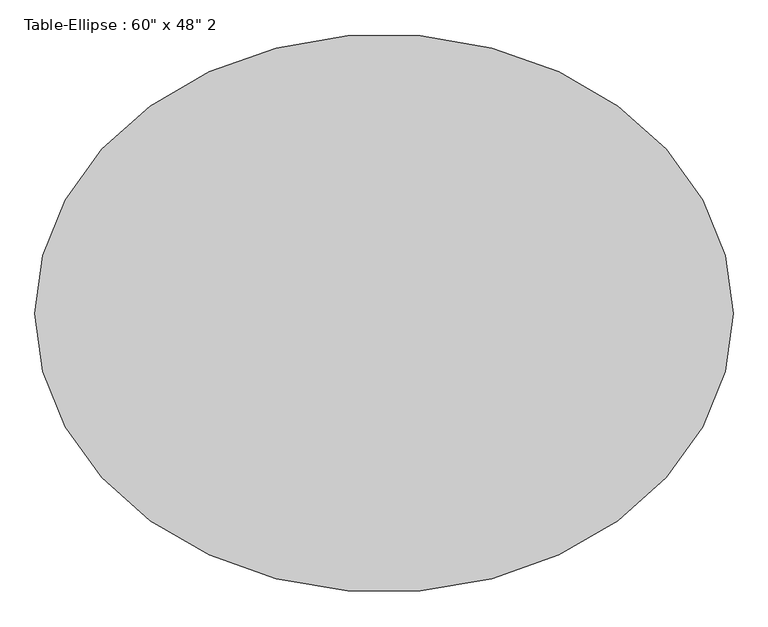
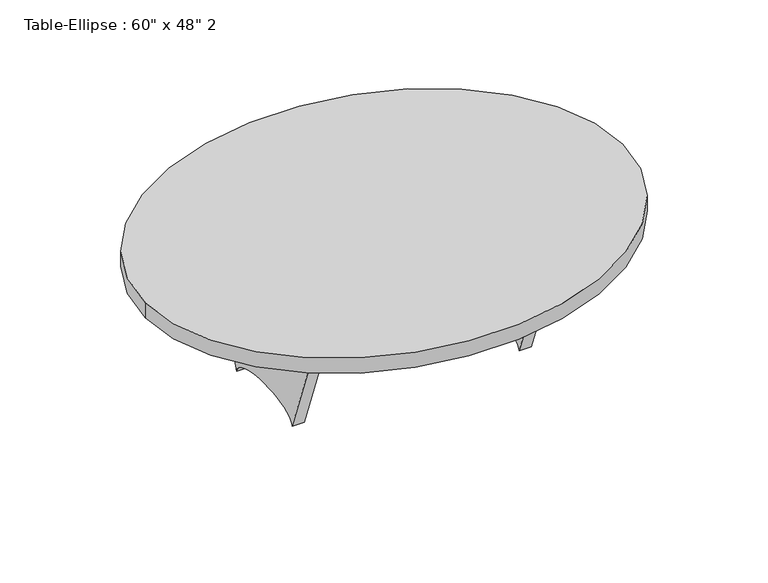
"""IFC4 building model written with IfcOpenShell, lengths in millimetres: furniture geometry."""

from ifc_helpers import new_model, si_unit, point, frame, origin, place, context, project, spatial, ellipse_curve, trimmed, source, transform, mapped, element, save
from ifc_brep_helpers import plane_surface, extruded_surface, advanced_brep


def furniture_c105135d(model_context):
    return source(origin(), model_context, "Body", "AdvancedBrep", [
        advanced_brep(
        [(-762.0, 0.0, 457.2), (762.0, 0.0, 457.2), (-762.0, 0.0, 406.4), (762.0, 0.0, 406.4)],
        [
            (0, 1, ellipse_curve(frame((0.0, 0.0, 457.2), z_axis=(0.0, 0.0, 1.0), x_axis=(1.0, 0.0, 0.0)), 762.0, 609.6)),
            (1, 0, ellipse_curve(frame((0.0, 0.0, 457.2), z_axis=(0.0, 0.0, 1.0), x_axis=(1.0, 0.0, 0.0)), 762.0, 609.6)),
            (2, 3, ellipse_curve(frame((0.0, 0.0, 406.4), z_axis=(0.0, 0.0, -1.0), x_axis=(1.0, 0.0, 0.0)), 762.0, 609.6)),
            (3, 2, ellipse_curve(frame((0.0, 0.0, 406.4), z_axis=(0.0, 0.0, -1.0), x_axis=(1.0, 0.0, 0.0)), 762.0, 609.6)),
            (0, 2),
            (3, 1),
        ],
        [
            plane_surface(frame((762.0, 0.0, 457.2), z_axis=(0.0, 0.0, 1.0), x_axis=(0.0, 1.0, 0.0))),
            plane_surface(frame((762.0, 0.0, 406.4), z_axis=(0.0, 0.0, -1.0), x_axis=(0.0, -1.0, 0.0))),
            extruded_surface(trimmed(ellipse_curve(frame((0.0, 0.0, 355.6), z_axis=(0.0, 0.0, 1.0), x_axis=(1.0, 0.0, 0.0)), 762.0, 609.6), [point((-762.0, 0.0, 355.6))], [point((762.0, 0.0, 355.6))], True, "CARTESIAN"), (0.0, 0.0, 50.799999999999955), 50.799999999999955),
            extruded_surface(trimmed(ellipse_curve(frame((0.0, 0.0, 355.6), z_axis=(0.0, 0.0, 1.0), x_axis=(1.0, 0.0, 0.0)), 762.0, 609.6), [point((762.0, 0.0, 355.6))], [point((-762.0, 0.0, 355.6))], True, "CARTESIAN"), (0.0, 0.0, 50.799999999999955), 50.799999999999955),
        ],
        [
            (0, [[1, 2]]),
            (1, [[3, 4]]),
            (2, [[-1, 5, -4, 6]]),
            (3, [[-2, -6, -3, -5]]),
        ],
    ),
        advanced_brep(
        [(-342.9, 304.8, 406.4), (-342.9, -304.8, 406.4), (-342.9, -152.4, 0.0), (-342.9, 152.4, 0.0), (-381.0, 304.8, 406.4), (-381.0, 152.4, 0.0), (-381.0, -152.4, 0.0), (-381.0, -304.8, 406.4)],
        [
            (0, 1),
            (1, 2),
            (2, 3, ellipse_curve(frame((-342.9, 0.0, 0.0), z_axis=(-1.0, 0.0, 0.0), x_axis=(0.0, 1.0, 0.0)), 152.4, 50.8)),
            (3, 0),
            (4, 5),
            (5, 6, ellipse_curve(frame((-381.0, 0.0, 0.0), z_axis=(1.0, 0.0, 0.0), x_axis=(0.0, 1.0, 0.0)), 152.4, 50.8)),
            (6, 7),
            (7, 4),
            (0, 4),
            (7, 1),
            (6, 2),
            (5, 3),
        ],
        [
            plane_surface(frame((-342.9, -304.8, 406.4), z_axis=(1.0, 0.0, 0.0), x_axis=(0.0, -1.0, 0.0))),
            plane_surface(frame((-381.0, -304.8, 406.4), z_axis=(-1.0, 0.0, 0.0), x_axis=(0.0, 1.0, 0.0))),
            plane_surface(frame((-342.9, 304.8, 406.4), z_axis=(0.0, 0.0, 1.0), x_axis=(-1.0, 0.0, 0.0))),
            plane_surface(frame((-342.9, -304.8, 406.4), z_axis=(0.0, -0.9363291775690403, -0.3511234415884029), x_axis=(-1.0, 0.0, 0.0))),
            extruded_surface(trimmed(ellipse_curve(frame((-419.1, 0.0, 0.0), z_axis=(-1.0, 0.0, 0.0), x_axis=(0.0, 1.0, 0.0)), 152.4, 50.8), [point((-419.1, -152.4, 0.0))], [point((-419.1, 152.4, 0.0))], True, "CARTESIAN"), (38.10000000000002, 0.0, 0.0), 38.10000000000002),
            plane_surface(frame((-342.9, 152.4, 0.0), z_axis=(0.0, 0.9363291775690458, -0.3511234415883884), x_axis=(-1.0, 0.0, 0.0))),
        ],
        [
            (0, [[1, 2, 3, 4]]),
            (1, [[5, 6, 7, 8]]),
            (2, [[-1, 9, -8, 10]]),
            (3, [[-2, -10, -7, 11]]),
            (4, [[-3, -11, -6, 12]]),
            (5, [[-4, -12, -5, -9]]),
        ],
    ),
        advanced_brep(
        [(381.0, 304.8, 406.4), (381.0, -304.8, 406.4), (381.0, -152.4, 0.0), (381.0, 152.4, 0.0), (342.9, 304.8, 406.4), (342.9, 152.4, 0.0), (342.9, -152.4, 0.0), (342.9, -304.8, 406.4)],
        [
            (0, 1),
            (1, 2),
            (2, 3, ellipse_curve(frame((381.0, 0.0, 0.0), z_axis=(-1.0, 0.0, 0.0), x_axis=(0.0, 1.0, 0.0)), 152.4, 50.8)),
            (3, 0),
            (4, 5),
            (5, 6, ellipse_curve(frame((342.9, 0.0, 0.0), z_axis=(1.0, 0.0, 0.0), x_axis=(0.0, 1.0, 0.0)), 152.4, 50.8)),
            (6, 7),
            (7, 4),
            (0, 4),
            (7, 1),
            (6, 2),
            (5, 3),
        ],
        [
            plane_surface(frame((381.0, -304.8, 406.4), z_axis=(1.0, 0.0, 0.0), x_axis=(0.0, -1.0, 0.0))),
            plane_surface(frame((342.9, -304.8, 406.4), z_axis=(-1.0, 0.0, 0.0), x_axis=(0.0, 1.0, 0.0))),
            plane_surface(frame((381.0, 304.8, 406.4), z_axis=(0.0, 0.0, 1.0), x_axis=(-1.0, 0.0, 0.0))),
            plane_surface(frame((381.0, -304.8, 406.4), z_axis=(0.0, -0.9363291775690407, -0.35112344158840214), x_axis=(-1.0, 0.0, 0.0))),
            extruded_surface(trimmed(ellipse_curve(frame((304.8, 0.0, 0.0), z_axis=(-1.0, 0.0, 0.0), x_axis=(0.0, 1.0, 0.0)), 152.4, 50.8), [point((304.8, -152.4, 0.0))], [point((304.8, 152.4, 0.0))], True, "CARTESIAN"), (38.099999999999966, 0.0, 0.0), 38.099999999999966),
            plane_surface(frame((381.0, 152.4, 0.0), z_axis=(0.0, 0.9363291775690474, -0.351123441588384), x_axis=(-1.0, 0.0, 0.0))),
        ],
        [
            (0, [[1, 2, 3, 4]]),
            (1, [[5, 6, 7, 8]]),
            (2, [[-1, 9, -8, 10]]),
            (3, [[-2, -10, -7, 11]]),
            (4, [[-3, -11, -6, 12]]),
            (5, [[-4, -12, -5, -9]]),
        ],
    ),
        advanced_brep(
        [(-342.9, 19.05, 406.4), (342.9, 19.05, 406.4), (342.9, 19.05, 270.9333333), (-342.9, 19.05, 270.9333333), (-342.9, -19.05, 406.4), (-342.9, -19.05, 270.9333333), (342.9, -19.05, 270.9333333), (342.9, -19.05, 406.4)],
        [
            (0, 1),
            (1, 2),
            (2, 3, ellipse_curve(frame((0.0, 19.05, 270.9333333), z_axis=(0.0, -1.0, 0.0), x_axis=(1.0, 0.0, 0.0)), 342.9, 101.6)),
            (3, 0),
            (4, 5),
            (5, 6, ellipse_curve(frame((0.0, -19.05, 270.9333333), z_axis=(0.0, 1.0, 0.0), x_axis=(1.0, 0.0, 0.0)), 342.9, 101.6)),
            (6, 7),
            (7, 4),
            (0, 4),
            (7, 1),
            (6, 2),
            (5, 3),
        ],
        [
            plane_surface(frame((-342.9, 19.05, 406.4), z_axis=(0.0, 1.0, 0.0), x_axis=(1.0, 0.0, 0.0))),
            plane_surface(frame((-342.9, -19.05, 406.4), z_axis=(0.0, -1.0, 0.0), x_axis=(-1.0, 0.0, 0.0))),
            plane_surface(frame((-342.9, 19.05, 406.4), z_axis=(0.0, 0.0, 1.0), x_axis=(0.0, -1.0, 0.0))),
            plane_surface(frame((342.9, 19.05, 406.4), z_axis=(1.0, 0.0, 0.0), x_axis=(0.0, -1.0, 0.0))),
            extruded_surface(trimmed(ellipse_curve(frame((0.0, -57.15, 270.9333333), z_axis=(0.0, -1.0, 0.0), x_axis=(1.0, 0.0, 0.0)), 342.9, 101.6), [point((342.9, -57.15, 270.9333333))], [point((-342.9, -57.15, 270.9333333))], True, "CARTESIAN"), (0.0, 38.099999999999994, 0.0), 38.099999999999994),
            plane_surface(frame((-342.9, 19.05, 270.9333333), z_axis=(-1.0, 0.0, 0.0), x_axis=(0.0, -1.0, 0.0))),
        ],
        [
            (0, [[1, 2, 3, 4]]),
            (1, [[5, 6, 7, 8]]),
            (2, [[-1, 9, -8, 10]]),
            (3, [[-2, -10, -7, 11]]),
            (4, [[-3, -11, -6, 12]]),
            (5, [[-4, -12, -5, -9]]),
        ],
    ),
    ])


if __name__ == "__main__":
    model = new_model("IFC4")
    model_context = context("Model", 3, world=origin())
    ifc_project = project(units=[si_unit("LENGTHUNIT", "METRE", prefix="MILLI")], contexts=[model_context])
    site = spatial("IfcSite", under=ifc_project)
    building = spatial("IfcBuilding", under=site)
    placement = place(None, origin())
    furniture_shape = furniture_c105135d(model_context)
    element("IfcFurniture", 1, ObjectType="Table-Ellipse : 60\" x 48\" 2", at=placement, inside=building, context=model_context, shape_type="MappedRepresentation", body=[
        mapped(furniture_shape, transform((0.0, 0.0, 0.0), x_axis=(1.0, 0.0, 0.0), y_axis=(0.0, 1.0, 0.0), z_axis=(0.0, 0.0, 1.0))),
    ])
    save(model, "model.ifc")

# Revit data of these elements
# Type "Table-Ellipse : 60\" x 48\" 2"
#   Assembly Code = "E2020200"
#   Half Width = 2' - 0"
#   Half Length = 2' - 6"
#   Height = 1' - 6"
#   Length = 5' - 0"
#   Width = 4' - 0"
#   Base Material = Birch
#   Top Material = Birch
#   Default Elevation = 0
# Element 1 (IfcFurniture, "Table-Ellipse : 60\" x 48\" 2")
#   Materials on its faces: "Birch"
# Materials
#   "Birch": class "Wood", colour RGB 224 178 126, transparency 0, Description = "Betula Alleghaniensis", Cost = 0
